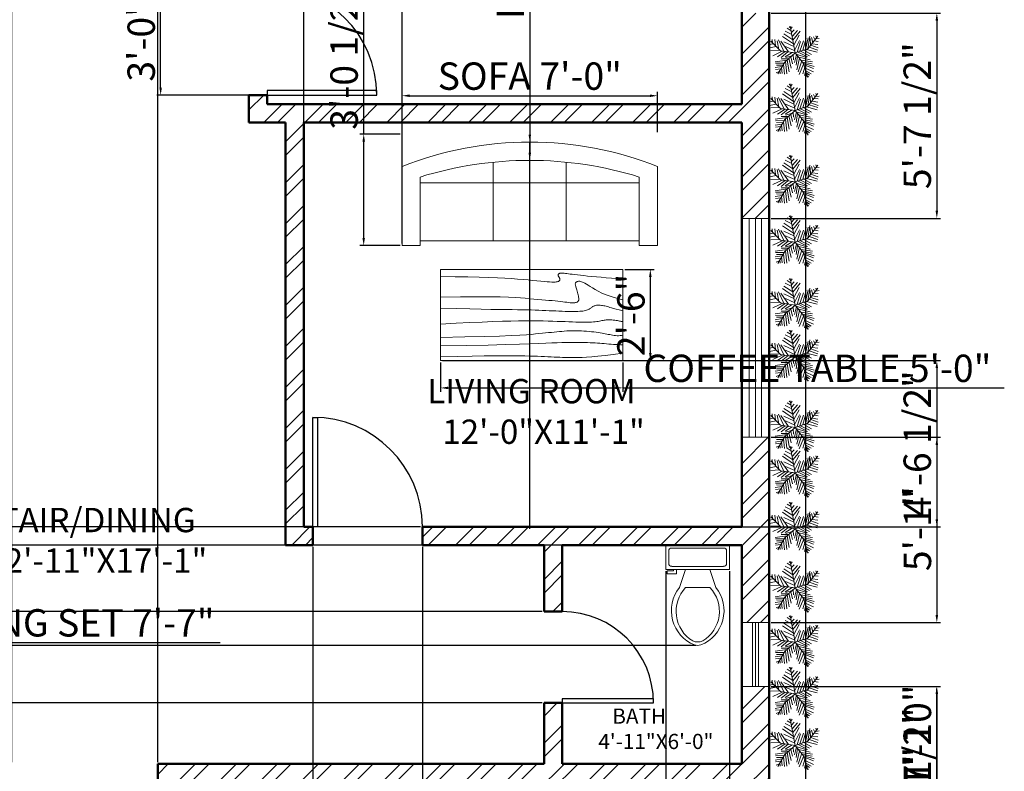
# Model space of a CAD drawing. Units: inches. Extents: x 176 to 806, y 915 to 1663.
# Tile 4 of 5: x 482 to 806, y 1198 to 1445. Entities that reach past the tile are written whole.
import ezdxf

# ---------------------------------------------------------------- set-up
doc = ezdxf.new("R2010")
doc.units = ezdxf.units.IN
for name, color, linetype, lineweight in [('A-ANNO-DIMS', 2, 'Continuous', 18), ('A-AREA-IDEN', 7, 'Continuous', 18), ('A-DOOR', 4, 'Continuous', 25), ('A-FLOR-FIXT', 9, 'Continuous', 18), ('A-FURN', 8, 'Continuous', 18), ('A-WALL', 7, 'Continuous', 50), ('A-WALL-PATT', 252, 'Continuous', 13), ('C-PROP', 8, 'Continuous', 25), ('L-PLNT', 3, 'Continuous', 13)]:
    doc.layers.add(name, color=color, linetype=linetype, lineweight=lineweight)
doc.layers.add('A-GLAZ', color=244, linetype='Continuous', lineweight=18, true_color=0x991b1e)
doc.styles.get("Standard").update_dxf_attribs({"font": 'arial.ttf'})
doc.dimstyles.new('ISO-25', dxfattribs={"dimtxt": 9, "dimasz": 2.5, "dimexe": 1.25, "dimexo": 0.625, "dimtad": 1, "dimlunit": 3, "dimtxsty": 'Standard', "dimcen": 2.5, "dimadec": 0, "dimazin": 0, "dimtfac": 1, "dimtmove": 0, "dimatfit": 3, "dimfxl": 1, "dimarcsym": 0})

# ---------------------------------------------------------------- blocks, each defined once
blk = doc.blocks.new('*U3')
for p, q in [((0, 0), (0, -6)), ((-40, 0), (-40, -6))]:
    blk.add_line(p, q)
blk.add_lwpolyline([(0, 0), (0, 40), (-1.75, 40), (-1.75, 0)], close=True)
blk.add_arc((0, 0), 40, 90, 180)
blk = doc.blocks.new('*U5')
for p, q in [((0, 0), (0, -6)), ((40, 0), (40, -6))]:
    blk.add_line(p, q)
blk.add_lwpolyline([(0, 0), (0, 40), (1.75, 40), (1.75, 0)], close=True)
blk.add_arc((0, 0), 40, 0, 90)
blk = doc.blocks.new('*U6')
for p, q in [((0, 0), (0, 6)), ((40, 0), (40, 6))]:
    blk.add_line(p, q)
blk.add_lwpolyline([(0, 0), (0, -40), (1.75, -40), (1.75, 0)], close=True)
blk.add_arc((0, 0), 40, 270, 0)
blk = doc.blocks.new('*U8')
for p, q in [((-7.288, 39.707), (-21.778, 46.673)), ((-8.737, 47.138), (-17.069, 52.711)), ((-10.186, 53.64), (-13.084, 55.962)), ((0, 0), (-10.5, 57)), ((-9.099, 51.782), (-6.563, 55.962)), ((-7.65, 43.423), (-2.578, 49.46)), ((-5.839, 35.992), (4.667, 48.067)), ((-5.114, 27.632), (10.463, 46.673)), ((-31.5, 4.5), (-52.5, 25.5)), ((-48.585, 21.131), (-49.309, 29.026)), ((-43.513, 28.561), (-42.427, 15.558)), ((-38.442, 26.239), (-34.819, 7.663)), ((-35.544, 28.097), (-24.314, 3.947)), ((-14.533, 2.09), (-30.834, 25.31)), ((-3.665, 19.273), (-27.574, 35.527)), ((-5.114, 28.097), (-24.676, 40.636)), ((-24.314, 23.917), (-2.941, 13.7)), ((-2.941, 16.486), (8.652, 37.85)), ((-1.129, 6.734), (9.014, 26.704)), ((3.942, 1.625), (11.187, 24.381)), ((10.101, 3.483), (17.708, 26.239)), ((16.259, 5.805), (23.142, 31.348)), ((22.055, 7.198), (27.489, 32.277)), ((27, 9), (48, 36)), ((27.127, 9.056), (31.112, 35.992)), ((31.836, 30.883), (32.561, 16.486)), ((35.096, 32.741), (37.27, 22.524)), ((38.719, 34.134), (41.979, 28.561)), ((40.53, 25.775), (48.862, 24.846)), ((43.791, 29.954), (51.036, 30.883)), ((44.153, 36.456), (45.239, 32.741)), ((-47.498, 19.737), (-55.83, 18.344)), ((-40.615, 13.7), (-55.105, 10.913)), ((-33.37, 6.269), (-52.207, 5.34)), ((-28.299, 3.483), (-47.86, -5.805)), ((-21.416, 3.018), (-38.079, -8.128)), ((0, 0), (-31.5, 4.5)), ((-15.982, 2.09), (-30.11, -9.521)), ((0, 0), (-22.5, -19.5)), ((-6.563, 1.161), (-21.416, -8.128)), ((-20.691, 13.7), (-1.129, 4.876)), ((0, 0), (27, 9)), ((0, 0), (18, -22.5)), ((6.478, 1.625), (26.04, -8.592)), ((11.187, 3.483), (30.749, -5.805)), ((18.07, 5.805), (35.096, -3.483)), ((24.229, 7.663), (46.688, 1.625)), ((29.662, 12.307), (48.137, 6.269)), ((33.285, 16.486), (48.862, 10.913)), ((36.183, 19.737), (48.137, 17.88)), ((-17.431, -15.094), (-42.789, -18.809)), ((-22.5, -19.5), (-37.5, -45)), ((-15.257, -12.772), (-30.11, -12.772)), ((-20.691, -18.345), (-17.793, -44.352)), ((-6.563, -5.805), (-19.967, -9.985)), ((-17.069, -15.094), (-12.721, -40.172)), ((-13.446, -11.378), (-8.737, -32.741)), ((-9.461, -8.592), (-6.201, -23.453)), ((-4.752, -3.483), (-3.665, -14.629)), ((2.493, -3.019), (-1.491, -20.202)), ((1.769, -2.555), (24.229, -9.521)), ((5.029, -6.27), (2.131, -25.775)), ((9.014, -11.378), (3.58, -35.992)), ((14.085, -16.951), (6.478, -40.172)), ((7.565, -9.056), (32.198, -14.629)), ((12.274, -15.094), (36.907, -18.809)), ((16.259, -19.738), (36.183, -22.989)), ((-28.299, -29.026), (-42.789, -31.348)), ((-24.314, -21.596), (-42.427, -22.06)), ((-30.834, -34.135), (-42.427, -35.528)), ((-34.457, -39.708), (-40.978, -42.494)), ((-26.849, -26.24), (-40.253, -25.775)), ((-32.646, -36.921), (-31.921, -44.352)), ((-29.023, -30.884), (-27.936, -43.887)), ((-25.038, -23.918), (-22.865, -45.281)), ((18.07, -22.524), (8.289, -45.745)), ((20.244, -30.419), (15.897, -44.816)), ((18, -22.5), (27, -52.5)), ((18.433, -22.524), (40.53, -29.026)), ((19.157, -25.311), (38.719, -33.206)), ((22.78, -37.85), (19.519, -48.532)), ((21.331, -32.741), (39.081, -40.636)), ((22.78, -38.314), (34.372, -44.816)), ((24.591, -45.745), (23.142, -50.854)), ((24.591, -43.423), (30.749, -47.603)), ((26.764, -49.925), (28.213, -50.854))]:
    blk.add_line(p, q)
blk = doc.blocks.new('*U13')
for p, q in [((9.5, -6), (9.5, -2)), ((-10, -8.5), (-8, -8.5)), ((-10, -9.5), (-10, -8.5)), ((-7, -9.5), (-10, -9.5)), ((-8, -8.5), (-8, -8)), ((-7, -8), (-7, -9.5)), ((-4, -8), (-6, -14)), ((4, -8), (6, -14)), ((4, -14), (-4, -14))]:
    blk.add_line(p, q)
blk.add_lwpolyline([(10.5, -8), (10.5, 0), (-10.5, 0), (-10.5, -8)], close=True)
for points in [[(-9.5, -2), (-9.5, -6)], [(8.5, -1), (-8.5, -1)], [(-8.5, -7), (8.5, -7)]]:
    blk.add_lwpolyline(points)
for centre, radius, start, end in [((-8.62, -1.88), 0.884, 81.8699, 188.1301), ((8.62, -1.88), 0.884, 351.8699, 98.1301), ((-8.62, -6.12), 0.884, 171.8699, 278.1301), ((8.62, -6.12), 0.884, 261.8699, 8.1301), ((3.52, -21.58), 12.17, 141.4691, 247.9714), ((4.2, -21.82), 11.33, 136.3677, 238.9468), ((-3.52, -21.58), 12.17, 292.0284, 38.5307), ((-4.2, -21.82), 11.33, 301.053, 43.6321), ((0, -27.88), 4, 245.7318, 294.2682), ((0, -29), 4, 254.8605, 285.1395)]:
    blk.add_arc(centre, radius, start, end)
blk = doc.blocks.new('Sofa - Roundback 7 ft.')
for p, q in [((-12.00002, -32.4421), (-12.00003, -6.5971)), ((11.99997, -32.4421), (11.99998, -6.5971)), ((-36.000027, -34), (-36.000027, -11.4696)), ((35.99998, -34), (35.99998, -11.4696)), ((-35.999844, -13.3819), (35.9998, -13.3819)), ((-36.000027, -32.4421), (35.99998, -32.4421))]:
    blk.add_line(p, q)
for points in [[(-36.000027, -34), (-42.000027, -34), (-42.000027, -8)], [(41.99998, -8), (41.99998, -34), (35.99998, -34)]]:
    blk.add_lwpolyline(points)
for centre, radius, start, end in [((0, -114.25), 114.25, 68.43141, 111.5686), ((-0.00001, -127.1968), 121.1968, 72.72033, 107.2797)]:
    blk.add_arc(centre, radius, start, end)
blk = doc.blocks.new('Table - Rectangular Woodgrain 60 x 30 in.')
for p, q in [((0, 0), (0, -30)), ((60, 0), (0, 0)), ((60, -30), (60, 0)), ((0, -30), (60, -30))]:
    blk.add_line(p, q)
for points in [[(0, -2.4), (4.8155, -2.418), (9.0302, -2.4688), (12.709, -2.5477), (15.9167, -2.65), (18.7181, -2.7711), (21.1781, -2.9063), (23.3616, -3.0508), (25.3333, -3.2), (27.1477, -3.3495), (28.8172, -3.4958), (30.3437, -3.636), (31.7291, -3.7667), (32.9756, -3.8849), (34.0849, -3.9875), (35.059, -4.0714), (35.9, -4.1334), (36.6114, -4.1711), (37.2041, -4.1854), (37.6906, -4.1779), (38.0833, -4.15), (38.3948, -4.1034), (38.6375, -4.0396), (38.8239, -3.9602), (38.9666, -3.8667), (39.0764, -3.7608), (39.1573, -3.6448), (39.2116, -3.521), (39.2416, -3.3917), (39.2498, -3.2593), (39.2385, -3.1261), (39.21, -2.9944), (39.1666, -2.8667), (39.111, -2.7447), (39.0468, -2.6281), (38.978, -2.5163), (38.9083, -2.4083), (38.8418, -2.3035), (38.7823, -2.201), (38.7337, -2.1001), (38.7, -2), (38.6844, -1.9003), (38.6875, -1.8021), (38.7094, -1.707), (38.75, -1.6167), (38.8094, -1.5326), (38.8875, -1.4563), (38.9844, -1.3893), (39.1, -1.3333), (39.2351, -1.2896), (39.3937, -1.2583), (39.5804, -1.2396), (39.8, -1.2333), (40.057, -1.2396), (40.3562, -1.2583), (40.7023, -1.2896), (41.1, -1.3333), (41.5547, -1.3895), (42.0755, -1.4573), (42.6721, -1.5361), (43.3542, -1.625), (44.1316, -1.7233), (45.014, -1.8302), (46.0114, -1.9449), (47.1333, -2.0667), (48.3862, -2.1947), (49.7625, -2.3281), (51.2513, -2.4663), (52.8416, -2.6083), (54.5226, -2.7535), (56.2833, -2.9011), (58.1127, -3.0501), (60, -3.2)], [(0, -9.2), (6.5759, -9.0858), (11.9385, -9.0365), (16.2527, -9.0418), (19.6833, -9.0917), (22.3952, -9.1759), (24.5531, -9.2844), (26.322, -9.4069), (27.8666, -9.5333), (29.3241, -9.6553), (30.7203, -9.7719), (32.0532, -9.8837), (33.3208, -9.9917), (34.5213, -10.0965), (35.6526, -10.199), (36.7128, -10.2999), (37.7, -10.4), (38.6129, -10.4996), (39.4531, -10.5969), (40.223, -10.6895), (40.925, -10.775), (41.5613, -10.8512), (42.1344, -10.9156), (42.6465, -10.966), (43.1, -11), (43.4976, -11.0158), (43.8437, -11.0136), (44.143, -10.9942), (44.4, -10.9583), (44.6195, -10.9069), (44.8062, -10.8406), (44.9648, -10.7603), (45.1, -10.6667), (45.2155, -10.5598), (45.3114, -10.4365), (45.3871, -10.2929), (45.4416, -10.125), (45.4743, -9.929), (45.4844, -9.7011), (45.4709, -9.4371), (45.4333, -9.1333), (45.3716, -8.7883), (45.2896, -8.4104), (45.1919, -8.0107), (45.0833, -7.6), (44.9685, -7.1893), (44.8521, -6.7896), (44.7388, -6.4117), (44.6333, -6.0667), (44.54, -5.7628), (44.4614, -5.4979), (44.4001, -5.2675), (44.3583, -5.0667), (44.3384, -4.8909), (44.3427, -4.7354), (44.3736, -4.5956), (44.4333, -4.4667), (44.5236, -4.3453), (44.6427, -4.2333), (44.7884, -4.1339), (44.9583, -4.05), (45.1501, -3.9849), (45.3614, -3.9417), (45.59, -3.9234), (45.8333, -3.9333), (46.0915, -3.9749), (46.3734, -4.0531), (46.6906, -4.1736), (47.0542, -4.3417), (47.4756, -4.5629), (47.9661, -4.8427), (48.5372, -5.1866), (49.2, -5.6), (49.9676, -6.0844), (50.8594, -6.625), (51.8965, -7.2031), (53.1, -7.8), (54.491, -8.3969), (56.0906, -8.975), (57.9199, -9.5156), (60, -10)], [(0, -12.8), (5.1847, -12.9322), (9.6213, -13.0323), (13.3963, -13.1059), (16.5958, -13.1583), (19.3063, -13.1952), (21.614, -13.2219), (23.6054, -13.2439), (25.3666, -13.2667), (26.9728, -13.2947), (28.4531, -13.3281), (29.8256, -13.3663), (31.1083, -13.4083), (32.3191, -13.4535), (33.476, -13.501), (34.597, -13.5501), (35.7, -13.6), (36.7984, -13.6497), (37.8875, -13.6979), (38.9578, -13.743), (40, -13.7833), (41.0047, -13.8174), (41.9625, -13.8438), (42.864, -13.8607), (43.7, -13.8667), (44.4631, -13.8604), (45.1552, -13.8417), (45.7801, -13.8104), (46.3416, -13.7667), (46.8439, -13.7104), (47.2906, -13.6417), (47.6858, -13.5604), (48.0333, -13.4667), (48.3375, -13.3608), (48.6042, -13.2448), (48.8396, -13.121), (49.05, -12.9917), (49.2417, -12.8593), (49.4208, -12.7261), (49.5937, -12.5944), (49.7667, -12.4667), (49.9452, -12.3451), (50.1323, -12.2313), (50.3303, -12.1268), (50.5416, -12.0333), (50.7686, -11.9524), (51.0135, -11.8854), (51.2788, -11.8341), (51.5666, -11.8), (51.8785, -11.7843), (52.2116, -11.7865), (52.562, -11.8059), (52.926, -11.8417), (53.2998, -11.8931), (53.6795, -11.9594), (54.0614, -12.0397), (54.4416, -12.1333), (54.8223, -12.2401), (55.2293, -12.3625), (55.6942, -12.5037), (56.2489, -12.6667), (56.9251, -12.8547), (57.7545, -13.0708), (58.7689, -13.3182), (60, -13.6)], [(0, -18), (5.124, -17.7273), (9.6609, -17.5057), (13.6705, -17.3303), (17.2125, -17.1958), (20.3467, -17.0973), (23.1328, -17.0297), (25.6307, -16.9878), (27.9, -16.9667), (29.9928, -16.9617), (31.9302, -16.9703), (33.7254, -16.9907), (35.3917, -17.0208), (36.9423, -17.0588), (38.3906, -17.1026), (39.7499, -17.1503), (41.0333, -17.2), (42.2519, -17.2496), (43.4073, -17.2969), (44.4986, -17.3395), (45.525, -17.375), (46.4858, -17.4012), (47.3802, -17.4156), (48.2074, -17.416), (48.9667, -17.4), (49.6583, -17.3662), (50.2872, -17.3167), (50.8595, -17.2547), (51.3812, -17.1833), (51.8584, -17.1057), (52.2971, -17.025), (52.7034, -16.9443), (53.0833, -16.8667), (53.443, -16.7951), (53.789, -16.7313), (54.128, -16.6768), (54.4666, -16.6334), (54.8115, -16.6024), (55.1693, -16.5854), (55.5465, -16.5841), (55.95, -16.6), (56.3828, -16.6337), (56.8346, -16.6823), (57.2915, -16.7418), (57.7396, -16.8084), (58.165, -16.878), (58.5539, -16.9469), (58.8924, -17.0111), (59.1666, -17.0667), (59.3679, -17.1107), (59.5078, -17.1438), (59.6032, -17.1675), (59.6708, -17.1833), (59.7275, -17.193), (59.7901, -17.1979), (59.8753, -17.1998), (60, -17.2)], [(0, -22.4), (8.0098, -22.2501), (14.4094, -22.1011), (19.4168, -21.9535), (23.25, -21.8083), (26.1269, -21.6663), (28.2656, -21.5281), (29.884, -21.3947), (31.2, -21.2667), (32.3967, -21.1448), (33.5172, -21.0292), (34.5697, -20.9198), (35.5625, -20.8167), (36.5037, -20.7198), (37.4015, -20.6292), (38.2642, -20.5448), (39.1, -20.4667), (39.9164, -20.3951), (40.7187, -20.3313), (41.5117, -20.2768), (42.3, -20.2333), (43.0883, -20.2024), (43.8812, -20.1854), (44.6836, -20.1841), (45.5, -20.2), (46.3328, -20.234), (47.1747, -20.2844), (48.0163, -20.3488), (48.8479, -20.425), (49.66, -20.5106), (50.4429, -20.6031), (51.1872, -20.7004), (51.8833, -20.8), (52.5246, -20.8999), (53.1166, -20.9995), (53.6681, -21.0983), (54.1875, -21.1958), (54.6834, -21.2919), (55.1646, -21.3859), (55.6394, -21.4777), (56.1167, -21.5667), (56.6028, -21.6515), (57.0961, -21.7266), (57.5929, -21.7852), (58.0896, -21.8208), (58.5823, -21.8268), (59.0674, -21.7964), (59.5412, -21.723), (60, -21.6)], [(0, -25.2), (8.6355, -25.0504), (15.7026, -24.9031), (21.4049, -24.7606), (25.9458, -24.625), (29.529, -24.4988), (32.3578, -24.3844), (34.6359, -24.284), (36.5667, -24.2), (38.3213, -24.1341), (39.9417, -24.0854), (41.437, -24.0523), (42.8167, -24.0333), (44.0901, -24.0268), (45.2667, -24.0313), (46.3557, -24.0451), (47.3667, -24.0667), (48.309, -24.0947), (49.1928, -24.1287), (50.0284, -24.168), (50.826, -24.2125), (51.5959, -24.2617), (52.3483, -24.3151), (53.0935, -24.3725), (53.8417, -24.4334), (54.6009, -24.497), (55.3699, -24.561), (56.1454, -24.6226), (56.9239, -24.6792), (57.7021, -24.7279), (58.4764, -24.7662), (59.2435, -24.7911), (60, -24.8)], [(0, -28.8), (5.6867, -28.6681), (10.45, -28.5698), (14.407, -28.5012), (17.675, -28.4584), (20.3711, -28.4374), (22.6125, -28.4344), (24.5164, -28.4455), (26.2, -28.4667), (27.762, -28.4947), (29.2276, -28.5281), (30.6033, -28.5663), (31.8958, -28.6084), (33.1118, -28.6535), (34.2578, -28.7011), (35.3405, -28.7501), (36.3666, -28.8), (37.3443, -28.8497), (38.288, -28.8974), (39.2137, -28.9412), (40.1375, -28.9792), (41.0753, -29.0093), (42.0432, -29.0297), (43.0572, -29.0384), (44.1333, -29.0333), (45.2936, -29.0114), (46.5843, -28.9641), (48.0579, -28.8816), (49.7666, -28.7542), (51.7629, -28.5721), (54.0989, -28.3255), (56.8272, -28.0048), (60, -27.6)]]:
    blk.add_lwpolyline(points)
blk = doc.blocks.new('WIN-GLAZING-72IN')
for p, q in [((0, 2), (72, 2)), ((0, 0), (72, 0)), ((0, -2), (72, -2))]:
    blk.add_line(p, q)
blk = doc.blocks.new('WIN-GLAZING-21IN')
for p, q in [((0, 1), (21, 1)), ((0, 0), (21, 0)), ((0, -1), (21, -1))]:
    blk.add_line(p, q)
blk = doc.blocks.new('*D34')
at = {"layer": 'A-ANNO-DIMS', "color": 0, "lineweight": -2, "transparency": 16777216}
for p, q in [((354.6, 1253.2), (354.6, 1238.92)), ((445.6, 1253.2), (445.6, 1238.92)), ((357.1, 1240.17), (443.1, 1240.17)), ((445.6, 1240.17), (548.27, 1240.17))]:
    blk.add_line(p, q, dxfattribs=at)
at = {"layer": 'A-ANNO-DIMS', "color": 0, "transparency": 16777216}
for points in [[(357.1, 1240.59), (357.1, 1239.75), (354.6, 1240.17)], [(443.1, 1240.59), (443.1, 1239.75), (445.6, 1240.17)]]:
    blk.add_solid(points, dxfattribs=at)
at = {"layer": 'Defpoints', "color": 0, "transparency": 16777216}
for p in [(354.6, 1253.82), (445.6, 1253.82), (445.6, 1240.17)]:
    blk.add_point(p, dxfattribs=at)
at = {"layer": 'A-ANNO-DIMS', "color": 0, "transparency": 16777216, "insert": (498.18, 1245.45), "char_height": 9, "attachment_point": 5}
blk.add_mtext('DINING SET 7\'-7"', dxfattribs=at)
blk = doc.blocks.new('*D36')
at = {"layer": 'A-ANNO-DIMS', "color": 0, "lineweight": -2, "transparency": 16777216}
for p, q in [((608.02, 1408.04), (608.02, 1421.26)), ((692.02, 1408.04), (692.02, 1421.26)), ((610.52, 1420.01), (689.52, 1420.01))]:
    blk.add_line(p, q, dxfattribs=at)
at = {"layer": 'A-ANNO-DIMS', "color": 0, "transparency": 16777216}
for points in [[(610.52, 1420.43), (610.52, 1419.59), (608.02, 1420.01)], [(689.52, 1420.43), (689.52, 1419.59), (692.02, 1420.01)]]:
    blk.add_solid(points, dxfattribs=at)
at = {"layer": 'Defpoints', "color": 0, "transparency": 16777216}
for p in [(692.02, 1420.01), (608.02, 1407.41), (692.02, 1407.41)]:
    blk.add_point(p, dxfattribs=at)
at = {"layer": 'A-ANNO-DIMS', "color": 0, "transparency": 16777216, "insert": (650.02, 1425.29), "char_height": 9, "attachment_point": 5}
blk.add_mtext('SOFA 7\'-0"', dxfattribs=at)
blk = doc.blocks.new('*D37')
at = {"layer": 'A-ANNO-DIMS', "color": 0, "lineweight": -2, "transparency": 16777216}
for p, q in [((595.42, 1407.41), (595.42, 1456.05)), ((607.4, 1407.41), (594.17, 1407.41)), ((595.42, 1373.24), (595.42, 1404.91)), ((607.4, 1370.74), (594.17, 1370.74))]:
    blk.add_line(p, q, dxfattribs=at)
at = {"layer": 'A-ANNO-DIMS', "color": 0, "transparency": 16777216}
for points in [[(595.01, 1404.91), (595.84, 1404.91), (595.42, 1407.41)], [(595.01, 1373.24), (595.84, 1373.24), (595.42, 1370.74)]]:
    blk.add_solid(points, dxfattribs=at)
at = {"layer": 'Defpoints', "color": 0, "transparency": 16777216}
for p in [(595.42, 1407.41), (608.02, 1407.41), (608.02, 1370.74)]:
    blk.add_point(p, dxfattribs=at)
at = {"layer": 'A-ANNO-DIMS', "color": 0, "transparency": 16777216, "insert": (590.14, 1432.98), "char_height": 9, "attachment_point": 5, "rotation": 90}
blk.add_mtext('3\'-0 1/2"', dxfattribs=at)
blk = doc.blocks.new('*D38')
at = {"layer": 'A-ANNO-DIMS', "color": 0, "lineweight": -2, "transparency": 16777216}
for p, q in [((620.66, 1332.28), (620.66, 1322.65)), ((680.66, 1332.28), (680.66, 1322.65)), ((623.16, 1323.9), (678.16, 1323.9)), ((680.66, 1323.9), (806.03, 1323.9))]:
    blk.add_line(p, q, dxfattribs=at)
at = {"layer": 'A-ANNO-DIMS', "color": 0, "transparency": 16777216}
for points in [[(623.16, 1324.32), (623.16, 1323.48), (620.66, 1323.9)], [(678.16, 1324.32), (678.16, 1323.48), (680.66, 1323.9)]]:
    blk.add_solid(points, dxfattribs=at)
at = {"layer": 'Defpoints', "color": 0, "transparency": 16777216}
for p in [(620.66, 1332.9), (680.66, 1332.9), (680.66, 1323.9)]:
    blk.add_point(p, dxfattribs=at)
at = {"layer": 'A-ANNO-DIMS', "color": 0, "transparency": 16777216, "insert": (744.59, 1329.18), "char_height": 9, "attachment_point": 5}
blk.add_mtext('COFFEE TABLE 5\'-0"', dxfattribs=at)
blk = doc.blocks.new('*D39')
at = {"layer": 'A-ANNO-DIMS', "color": 0, "lineweight": -2, "transparency": 16777216}
for p, q in [((681.28, 1362.9), (690.91, 1362.9)), ((689.66, 1335.4), (689.66, 1360.4)), ((681.28, 1332.9), (690.91, 1332.9))]:
    blk.add_line(p, q, dxfattribs=at)
at = {"layer": 'A-ANNO-DIMS', "color": 0, "transparency": 16777216}
for points in [[(689.24, 1360.4), (690.07, 1360.4), (689.66, 1362.9)], [(689.24, 1335.4), (690.07, 1335.4), (689.66, 1332.9)]]:
    blk.add_solid(points, dxfattribs=at)
at = {"layer": 'Defpoints', "color": 0, "transparency": 16777216}
for p in [(680.66, 1362.9), (689.66, 1362.9), (680.66, 1332.9)]:
    blk.add_point(p, dxfattribs=at)
at = {"layer": 'A-ANNO-DIMS', "color": 0, "transparency": 16777216, "insert": (684.44, 1347.9), "char_height": 9, "attachment_point": 5, "rotation": 90}
blk.add_mtext('2\'-6"', dxfattribs=at)
blk = doc.blocks.new('*D45')
at = {"layer": 'A-ANNO-DIMS', "color": 0, "lineweight": -2, "transparency": 16777216}
for p, q in [((729.33, 1447.21), (785.1, 1447.21)), ((783.85, 1444.71), (783.85, 1382.17)), ((729.33, 1379.67), (785.1, 1379.67))]:
    blk.add_line(p, q, dxfattribs=at)
at = {"layer": 'A-ANNO-DIMS', "color": 0, "transparency": 16777216}
for points in [[(783.43, 1444.71), (784.27, 1444.71), (783.85, 1447.21)], [(783.43, 1382.17), (784.27, 1382.17), (783.85, 1379.67)]]:
    blk.add_solid(points, dxfattribs=at)
at = {"layer": 'Defpoints', "color": 0, "transparency": 16777216}
for p in [(728.7, 1447.21), (728.7, 1379.67), (783.85, 1379.67)]:
    blk.add_point(p, dxfattribs=at)
at = {"layer": 'A-ANNO-DIMS', "color": 0, "transparency": 16777216, "insert": (778.57, 1413.44), "char_height": 9, "attachment_point": 5, "rotation": 90}
blk.add_mtext('5\'-7 1/2"', dxfattribs=at)
blk = doc.blocks.new('*D46')
at = {"layer": 'A-ANNO-DIMS', "color": 0, "lineweight": -2, "transparency": 16777216}
for p, q in [((729.33, 1307.67), (785.1, 1307.67)), ((783.85, 1305.17), (783.85, 1249.21)), ((729.33, 1246.71), (785.1, 1246.71))]:
    blk.add_line(p, q, dxfattribs=at)
at = {"layer": 'A-ANNO-DIMS', "color": 0, "transparency": 16777216}
for points in [[(783.43, 1305.17), (784.27, 1305.17), (783.85, 1307.67)], [(783.43, 1249.21), (784.27, 1249.21), (783.85, 1246.71)]]:
    blk.add_solid(points, dxfattribs=at)
at = {"layer": 'Defpoints', "color": 0, "transparency": 16777216}
for p in [(728.7, 1307.67), (728.7, 1246.71), (783.85, 1246.71)]:
    blk.add_point(p, dxfattribs=at)
at = {"layer": 'A-ANNO-DIMS', "color": 0, "transparency": 16777216, "insert": (778.63, 1277.19), "char_height": 9, "attachment_point": 5, "rotation": 90}
blk.add_mtext('5\'-1"', dxfattribs=at)
blk = doc.blocks.new('*D47')
at = {"layer": 'A-ANNO-DIMS', "color": 0, "lineweight": -2, "transparency": 16777216}
for p, q in [((729.33, 1225.71), (785.1, 1225.71)), ((783.85, 1223.21), (783.85, 1161.23)), ((729.33, 1158.73), (785.1, 1158.73))]:
    blk.add_line(p, q, dxfattribs=at)
at = {"layer": 'A-ANNO-DIMS', "color": 0, "transparency": 16777216}
for points in [[(783.43, 1223.21), (784.27, 1223.21), (783.85, 1225.71)], [(783.43, 1161.23), (784.27, 1161.23), (783.85, 1158.73)]]:
    blk.add_solid(points, dxfattribs=at)
at = {"layer": 'Defpoints', "color": 0, "transparency": 16777216}
for p in [(728.7, 1225.71), (728.7, 1158.73), (783.85, 1158.73)]:
    blk.add_point(p, dxfattribs=at)
at = {"layer": 'A-ANNO-DIMS', "color": 0, "transparency": 16777216, "insert": (778.65, 1192.22), "char_height": 9, "attachment_point": 5, "rotation": 90}
blk.add_mtext('5\'-7"', dxfattribs=at)
blk = doc.blocks.new('*D52')
at = {"layer": 'A-ANNO-DIMS', "color": 0, "lineweight": -2, "transparency": 16777216}
for p, q in [((479.7, 1200.83), (479.7, 1645.51)), ((527.7, 1200.83), (527.7, 1645.51)), ((482.2, 1644.26), (525.2, 1644.26))]:
    blk.add_line(p, q, dxfattribs=at)
at = {"layer": 'A-ANNO-DIMS', "color": 0, "transparency": 16777216}
for points in [[(482.2, 1644.67), (482.2, 1643.84), (479.7, 1644.26)], [(525.2, 1644.67), (525.2, 1643.84), (527.7, 1644.26)]]:
    blk.add_solid(points, dxfattribs=at)
at = {"layer": 'Defpoints', "color": 0, "transparency": 16777216}
for p in [(527.7, 1644.26), (479.7, 1200.21), (527.7, 1200.21)]:
    blk.add_point(p, dxfattribs=at)
at = {"layer": 'A-ANNO-DIMS', "color": 0, "transparency": 16777216, "insert": (503.7, 1649.48), "char_height": 9, "attachment_point": 5}
blk.add_mtext('4\'-0"', dxfattribs=at)
blk = doc.blocks.new('*D54')
at = {"layer": 'A-ANNO-DIMS', "color": 0, "lineweight": -2, "transparency": 16777216}
for p, q in [((247.1, 1280.71), (247.1, 1283.21)), ((614.08, 1278.21), (245.85, 1278.21)), ((247.1, 1278.21), (247.1, 1272.21)), ((614.08, 1272.21), (245.85, 1272.21)), ((247.1, 1269.71), (247.1, 1242.03))]:
    blk.add_line(p, q, dxfattribs=at)
at = {"layer": 'A-ANNO-DIMS', "color": 0, "transparency": 16777216}
for points in [[(246.68, 1280.71), (247.52, 1280.71), (247.1, 1278.21)], [(246.68, 1269.71), (247.52, 1269.71), (247.1, 1272.21)]]:
    blk.add_solid(points, dxfattribs=at)
at = {"layer": 'Defpoints', "color": 0, "transparency": 16777216}
for p in [(614.7, 1278.21), (247.1, 1272.21), (614.7, 1272.21)]:
    blk.add_point(p, dxfattribs=at)
at = {"layer": 'A-ANNO-DIMS', "color": 0, "transparency": 16777216, "insert": (241.88, 1254.62), "char_height": 9, "attachment_point": 5, "rotation": 90}
blk.add_mtext('0\'-6"', dxfattribs=at)
blk = doc.blocks.new('*D58')
at = {"layer": 'A-ANNO-DIMS', "color": 0, "lineweight": -2, "transparency": 16777216}
for p, q in [((654.08, 1250.31), (245.85, 1250.31)), ((247.1, 1222.81), (247.1, 1247.81)), ((654.08, 1220.31), (245.85, 1220.31))]:
    blk.add_line(p, q, dxfattribs=at)
at = {"layer": 'A-ANNO-DIMS', "color": 0, "transparency": 16777216}
for points in [[(246.68, 1247.81), (247.52, 1247.81), (247.1, 1250.31)], [(246.68, 1222.81), (247.52, 1222.81), (247.1, 1220.31)]]:
    blk.add_solid(points, dxfattribs=at)
at = {"layer": 'Defpoints', "color": 0, "transparency": 16777216}
for p in [(247.1, 1250.31), (654.7, 1250.31), (654.7, 1220.31)]:
    blk.add_point(p, dxfattribs=at)
at = {"layer": 'A-ANNO-DIMS', "color": 0, "transparency": 16777216, "insert": (241.88, 1235.31), "char_height": 9, "attachment_point": 5, "rotation": 90}
blk.add_mtext('2\'-6"', dxfattribs=at)
blk = doc.blocks.new('*D60')
at = {"layer": 'A-ANNO-DIMS', "color": 0, "lineweight": -2, "transparency": 16777216}
for p, q in [((578.7, 1271.58), (578.7, 983.8)), ((614.7, 1271.58), (614.7, 983.8)), ((581.2, 985.05), (612.2, 985.05))]:
    blk.add_line(p, q, dxfattribs=at)
at = {"layer": 'A-ANNO-DIMS', "color": 0, "transparency": 16777216}
for points in [[(581.2, 985.47), (581.2, 984.64), (578.7, 985.05)], [(612.2, 985.47), (612.2, 984.64), (614.7, 985.05)]]:
    blk.add_solid(points, dxfattribs=at)
at = {"layer": 'Defpoints', "color": 0, "transparency": 16777216}
for p in [(578.7, 1272.21), (614.7, 1272.21), (614.7, 985.05)]:
    blk.add_point(p, dxfattribs=at)
at = {"layer": 'A-ANNO-DIMS', "color": 0, "transparency": 16777216, "insert": (596.7, 990.28), "char_height": 9, "attachment_point": 5}
blk.add_mtext('3\'-0"', dxfattribs=at)
blk = doc.blocks.new('*D63')
at = {"layer": 'A-ANNO-DIMS', "color": 0, "lineweight": -2, "transparency": 16777216}
for p, q in [((783.85, 1169.12), (783.85, 1217.75)), ((334.37, 1169.12), (785.1, 1169.12)), ((783.85, 1129.89), (783.85, 1166.62)), ((334.37, 1127.39), (785.1, 1127.39))]:
    blk.add_line(p, q, dxfattribs=at)
at = {"layer": 'A-ANNO-DIMS', "color": 0, "transparency": 16777216}
for points in [[(783.43, 1166.62), (784.27, 1166.62), (783.85, 1169.12)], [(783.43, 1129.89), (784.27, 1129.89), (783.85, 1127.39)]]:
    blk.add_solid(points, dxfattribs=at)
at = {"layer": 'Defpoints', "color": 0, "transparency": 16777216}
for p in [(333.74, 1169.12), (783.85, 1169.12), (333.74, 1127.39)]:
    blk.add_point(p, dxfattribs=at)
at = {"layer": 'A-ANNO-DIMS', "color": 0, "transparency": 16777216, "insert": (778.57, 1194.68), "char_height": 9, "attachment_point": 5, "rotation": 90}
blk.add_mtext('3\'-5 1/2"', dxfattribs=at)
blk = doc.blocks.new('*D64')
at = {"layer": 'A-ANNO-DIMS', "color": 0, "lineweight": -2, "transparency": 16777216}
for p, q in [((563.08, 1456.21), (527.4, 1456.21)), ((528.65, 1422.71), (528.65, 1453.71)), ((563.08, 1420.21), (527.4, 1420.21))]:
    blk.add_line(p, q, dxfattribs=at)
at = {"layer": 'A-ANNO-DIMS', "color": 0, "transparency": 16777216}
for points in [[(528.24, 1453.71), (529.07, 1453.71), (528.65, 1456.21)], [(528.24, 1422.71), (529.07, 1422.71), (528.65, 1420.21)]]:
    blk.add_solid(points, dxfattribs=at)
at = {"layer": 'Defpoints', "color": 0, "transparency": 16777216}
for p in [(528.65, 1456.21), (563.7, 1456.21), (563.7, 1420.21)]:
    blk.add_point(p, dxfattribs=at)
at = {"layer": 'A-ANNO-DIMS', "color": 0, "transparency": 16777216, "insert": (523.43, 1438.21), "char_height": 9, "attachment_point": 5, "rotation": 90}
blk.add_mtext('3\'-0"', dxfattribs=at)
blk = doc.blocks.new('*D65')
at = {"layer": 'A-ANNO-DIMS', "color": 0, "lineweight": -2, "transparency": 16777216}
for p, q in [((575.7, 1278.83), (575.7, 1645.51)), ((608.02, 1371.37), (608.02, 1645.51)), ((575.7, 1644.26), (526.9, 1644.26)), ((605.52, 1644.26), (578.2, 1644.26))]:
    blk.add_line(p, q, dxfattribs=at)
at = {"layer": 'A-ANNO-DIMS', "color": 0, "transparency": 16777216}
for points in [[(578.2, 1644.67), (578.2, 1643.84), (575.7, 1644.26)], [(605.52, 1644.67), (605.52, 1643.84), (608.02, 1644.26)]]:
    blk.add_solid(points, dxfattribs=at)
at = {"layer": 'Defpoints', "color": 0, "transparency": 16777216}
for p in [(575.7, 1644.26), (608.02, 1370.74), (575.7, 1278.21)]:
    blk.add_point(p, dxfattribs=at)
at = {"layer": 'A-ANNO-DIMS', "color": 0, "transparency": 16777216, "insert": (550.05, 1649.53), "char_height": 9, "attachment_point": 5}
blk.add_mtext('2\'-8 1/2"', dxfattribs=at)
blk = doc.blocks.new('*D66')
at = {"layer": 'A-ANNO-DIMS', "color": 0, "lineweight": -2, "transparency": 16777216}
for p, q in [((621.28, 1332.9), (785.1, 1332.9)), ((783.85, 1330.4), (783.85, 1280.71)), ((615.33, 1278.21), (785.1, 1278.21))]:
    blk.add_line(p, q, dxfattribs=at)
at = {"layer": 'A-ANNO-DIMS', "color": 0, "transparency": 16777216}
for points in [[(783.43, 1330.4), (784.27, 1330.4), (783.85, 1332.9)], [(783.43, 1280.71), (784.27, 1280.71), (783.85, 1278.21)]]:
    blk.add_solid(points, dxfattribs=at)
at = {"layer": 'Defpoints', "color": 0, "transparency": 16777216}
for p in [(620.66, 1332.9), (614.7, 1278.21), (783.85, 1278.21)]:
    blk.add_point(p, dxfattribs=at)
at = {"layer": 'A-ANNO-DIMS', "color": 0, "transparency": 16777216, "insert": (778.57, 1305.55), "char_height": 9, "attachment_point": 5, "rotation": 90}
blk.add_mtext('4\'-6 1/2"', dxfattribs=at)
blk = doc.blocks.new('*D67')
at = {"layer": 'A-ANNO-DIMS', "color": 0, "lineweight": -2, "transparency": 16777216}
for p, q in [((783.85, 1191.21), (783.85, 1225.03)), ((336.33, 1191.21), (785.1, 1191.21)), ((783.85, 1171.62), (783.85, 1188.71)), ((334.37, 1169.12), (785.1, 1169.12))]:
    blk.add_line(p, q, dxfattribs=at)
at = {"layer": 'A-ANNO-DIMS', "color": 0, "transparency": 16777216}
for points in [[(783.43, 1188.71), (784.27, 1188.71), (783.85, 1191.21)], [(783.43, 1171.62), (784.27, 1171.62), (783.85, 1169.12)]]:
    blk.add_solid(points, dxfattribs=at)
at = {"layer": 'Defpoints', "color": 0, "transparency": 16777216}
for p in [(335.7, 1191.21), (783.85, 1191.21), (333.74, 1169.12)]:
    blk.add_point(p, dxfattribs=at)
at = {"layer": 'A-ANNO-DIMS', "color": 0, "transparency": 16777216, "insert": (778.63, 1209.37), "char_height": 9, "attachment_point": 5, "rotation": 90}
blk.add_mtext('1\'-10"', dxfattribs=at)
blk = doc.blocks.new('*D70')
at = {"layer": 'A-ANNO-DIMS', "color": 0, "lineweight": -2, "transparency": 16777216}
for p, q in [((694.73, 1263.58), (694.73, 983.8)), ((715.73, 1263.58), (715.73, 983.8)), ((697.23, 985.05), (713.23, 985.05)), ((715.73, 985.05), (742.56, 985.05))]:
    blk.add_line(p, q, dxfattribs=at)
at = {"layer": 'A-ANNO-DIMS', "color": 0, "transparency": 16777216}
for points in [[(697.23, 985.47), (697.23, 984.64), (694.73, 985.05)], [(713.23, 985.47), (713.23, 984.64), (715.73, 985.05)]]:
    blk.add_solid(points, dxfattribs=at)
at = {"layer": 'Defpoints', "color": 0, "transparency": 16777216}
for p in [(694.73, 1264.21), (715.73, 1264.21), (715.73, 985.05)]:
    blk.add_point(p, dxfattribs=at)
at = {"layer": 'A-ANNO-DIMS', "color": 0, "transparency": 16777216, "insert": (730.4, 990.27), "char_height": 9, "attachment_point": 5}
blk.add_mtext('1\'-9"', dxfattribs=at)
blk = doc.blocks.new('*D71')
at = {"layer": 'A-ANNO-DIMS', "color": 0, "lineweight": -2, "transparency": 16777216}
for p, q in [((715.11, 1272.21), (245.85, 1272.21)), ((247.1, 1269.71), (247.1, 1241.71)), ((704.61, 1239.21), (245.85, 1239.21))]:
    blk.add_line(p, q, dxfattribs=at)
at = {"layer": 'A-ANNO-DIMS', "color": 0, "transparency": 16777216}
for points in [[(246.68, 1269.71), (247.52, 1269.71), (247.1, 1272.21)], [(246.68, 1241.71), (247.52, 1241.71), (247.1, 1239.21)]]:
    blk.add_solid(points, dxfattribs=at)
at = {"layer": 'Defpoints', "color": 0, "transparency": 16777216}
for p in [(715.73, 1272.21), (247.1, 1239.21), (705.23, 1239.21)]:
    blk.add_point(p, dxfattribs=at)
at = {"layer": 'A-ANNO-DIMS', "color": 0, "transparency": 16777216, "insert": (241.88, 1255.71), "char_height": 9, "attachment_point": 5, "rotation": 90}
blk.add_mtext('2\'-9"', dxfattribs=at)
blk = doc.blocks.new('*D74')
at = {"layer": 'A-ANNO-DIMS', "color": 0, "lineweight": -2, "transparency": 16777216}
for p, q in [((650.03, 1491.85), (650.02, 1401.24)), ((650.02, 1277.55), (650.02, 1398.74))]:
    blk.add_line(p, q, dxfattribs=at)
at = {"layer": 'A-ANNO-DIMS', "color": 0, "transparency": 16777216}
blk.add_solid([(649.61, 1401.24), (650.44, 1401.24), (650.02, 1398.74)], dxfattribs=at)
at = {"layer": 'Defpoints', "color": 0, "transparency": 16777216}
for p in [(650.02, 1398.74), (650.02, 1277.55)]:
    blk.add_point(p, dxfattribs=at)
at = {"layer": 'A-ANNO-DIMS', "color": 0, "transparency": 16777216, "insert": (644.81, 1471.46), "char_height": 9, "attachment_point": 5, "rotation": 89.9999}
blk.add_mtext('R10\'-1"', dxfattribs=at)
blk = doc.blocks.new('*D75')
at = {"layer": 'A-ANNO-DIMS', "color": 0, "lineweight": -2, "transparency": 16777216}
for p, q in [((650.03, 1500.67), (650.02, 1407.24)), ((650.02, 1290.49), (650.02, 1404.74))]:
    blk.add_line(p, q, dxfattribs=at)
at = {"layer": 'A-ANNO-DIMS', "color": 0, "transparency": 16777216}
blk.add_solid([(649.61, 1407.24), (650.44, 1407.24), (650.02, 1404.74)], dxfattribs=at)
at = {"layer": 'Defpoints', "color": 0, "transparency": 16777216}
for p in [(650.02, 1404.74), (650.02, 1290.49)]:
    blk.add_point(p, dxfattribs=at)
at = {"layer": 'A-ANNO-DIMS', "color": 0, "transparency": 16777216, "insert": (644.75, 1473.29), "char_height": 9, "attachment_point": 5, "rotation": 89.9998}
blk.add_mtext('R9\'-6 1/2"', dxfattribs=at)

msp = doc.modelspace()

# ---------------------------------------------------------------- hatches: boundary and pattern name
at = {"layer": 'A-WALL-PATT'}
h = msp.add_hatch(dxfattribs=at)
h.set_pattern_fill('ANSI32', color=256)
h.paths.add_polyline_path([(302.704, 1050.206), (353.704, 1050.206), (353.704, 1059.206), (311.704, 1059.206), (311.704, 1191.206), (428.704, 1191.206), (428.704, 1200.206), (311.704, 1200.206), (311.704, 1357.206), (473.704, 1357.206), (473.704, 1363.206), (408.704, 1363.206), (408.704, 1366.206), (402.704, 1366.206), (402.704, 1363.206), (311.704, 1363.206), (311.704, 1376.706), (302.704, 1376.706)])
h.paths.add_polyline_path([(311.704, 1447.206), (302.704, 1447.206), (302.704, 1397.706), (311.704, 1397.706), (311.704, 1411.206), (402.704, 1411.206), (402.704, 1396.206), (408.704, 1396.206), (408.704, 1411.206), (473.704, 1411.206), (473.704, 1420.206), (467.704, 1420.206), (467.704, 1417.206), (311.704, 1417.206)])
h.paths.add_polyline_path([(467.704, 1059.206), (425.704, 1059.206), (425.704, 1050.206), (476.704, 1050.206), (476.704, 1191.206), (479.704, 1191.206), (479.704, 1200.206), (464.704, 1200.206), (464.704, 1191.206), (467.704, 1191.206)])
h.paths.add_polyline_path([(719.704, 1278.206), (614.704, 1278.206), (614.704, 1272.206), (654.704, 1272.206), (654.704, 1250.311), (660.704, 1250.311), (660.704, 1272.206), (719.704, 1272.206), (719.704, 1246.706), (728.704, 1246.706), (728.704, 1307.669), (719.704, 1307.669)])
h.paths.add_polyline_path([(728.704, 1447.206), (719.704, 1447.206), (719.704, 1417.206), (563.704, 1417.206), (563.704, 1420.206), (557.704, 1420.206), (557.704, 1411.206), (569.704, 1411.206), (569.704, 1272.206), (578.704, 1272.206), (578.704, 1278.206), (575.704, 1278.206), (575.704, 1411.206), (719.704, 1411.206), (719.704, 1379.669), (728.704, 1379.669)])
h.paths.add_polyline_path([(677.704, 1558.206), (677.704, 1549.206), (719.704, 1549.206), (719.704, 1519.206), (728.704, 1519.206), (728.704, 1558.206)])
h.paths.add_polyline_path([(526.204, 1558.206), (526.204, 1549.206), (557.704, 1549.206), (557.704, 1481.206), (554.704, 1481.206), (554.704, 1475.206), (557.704, 1475.206), (557.704, 1456.206), (563.704, 1456.206), (563.704, 1549.206), (605.704, 1549.206), (605.704, 1558.206)])
h.paths.add_polyline_path([(425.704, 1558.206), (425.704, 1549.206), (467.704, 1549.206), (467.704, 1456.206), (473.704, 1456.206), (473.704, 1475.206), (524.704, 1475.206), (524.704, 1481.206), (473.704, 1481.206), (473.704, 1549.206), (505.204, 1549.206), (505.204, 1558.206)])
h.paths.add_polyline_path([(311.704, 1549.206), (353.704, 1549.206), (353.704, 1558.206), (302.704, 1558.206), (302.704, 1519.206), (311.704, 1519.206)])
h = msp.add_hatch(dxfattribs=at)
h.set_pattern_fill('ANSI32', color=256)
h.paths.add_polyline_path([(719.704, 1200.206), (660.704, 1200.206), (660.704, 1220.311), (656.204, 1220.311), (654.704, 1220.311), (654.704, 1200.206), (527.704, 1200.206), (527.704, 1191.206), (728.704, 1191.206), (728.704, 1225.706), (719.704, 1225.706)])

# ---------------------------------------------------------------- linework, layer by layer
at = {"layer": 'A-GLAZ'}
for points in [[(728.704, 1379.669), (728.704, 1307.669), (719.704, 1307.669), (719.704, 1379.669)], [(728.704, 1246.706), (728.704, 1225.706), (719.704, 1225.706), (719.704, 1246.706)]]:
    msp.add_lwpolyline(points, close=True, dxfattribs=at)
at = {"layer": 'A-WALL'}
for p, q in [((728.704, 1558.206), (728.704, 1050.206)), ((719.704, 1549.206), (719.704, 1417.206)), ((563.704, 1420.206), (557.704, 1420.206)), ((557.704, 1420.206), (557.704, 1411.206)), ((563.704, 1420.206), (563.704, 1417.206)), ((563.704, 1417.206), (719.704, 1417.206)), ((557.704, 1411.206), (569.704, 1411.206)), ((569.704, 1411.206), (569.704, 1272.206)), ((575.704, 1411.206), (575.704, 1278.206)), ((575.704, 1411.206), (719.704, 1411.206)), ((719.704, 1411.206), (719.704, 1278.206)), ((575.704, 1278.206), (578.704, 1278.206)), ((578.704, 1278.206), (578.704, 1272.206)), ((614.704, 1278.206), (614.704, 1272.206)), ((614.704, 1278.206), (719.704, 1278.206)), ((569.704, 1272.206), (578.704, 1272.206)), ((614.704, 1272.206), (654.704, 1272.206)), ((654.704, 1272.206), (654.704, 1250.311)), ((660.704, 1272.206), (660.704, 1250.311)), ((660.704, 1272.206), (719.704, 1272.206)), ((719.704, 1272.206), (719.704, 1200.206)), ((660.704, 1250.311), (654.704, 1250.311)), ((660.704, 1220.311), (654.704, 1220.311)), ((654.704, 1220.311), (654.704, 1200.206)), ((660.704, 1220.311), (660.704, 1200.206)), ((527.704, 1191.206), (527.704, 1200.206)), ((527.704, 1200.206), (654.704, 1200.206)), ((660.704, 1200.206), (719.704, 1200.206))]:
    msp.add_line(p, q, dxfattribs=at)
at = {"layer": 'C-PROP'}
msp.add_line((740.704, 1570.206), (740.704, 1023.206), dxfattribs=at)

# ---------------------------------------------------------------- block references
at = {"layer": 'A-DOOR'}
for name, p, xscale, yscale, zscale, rotation in [('*U3', (563.704, 1420.206), 0.9, 0.9, 0.9, 269.9999999999985), ('*U6', (660.704, 1220.311), 0.7500000000000071, 0.7500000000000071, 0.7500000000000071, 90)]:
    msp.add_blockref(name, p, dxfattribs=dict(at, xscale=xscale, yscale=yscale, zscale=zscale, rotation=rotation))
at = {"layer": 'A-DOOR', "xscale": 0.9, "yscale": 0.9, "zscale": 0.9}
msp.add_blockref('*U5', (578.704, 1278.206), dxfattribs=at)
at = {"layer": 'A-FLOR-FIXT'}
msp.add_blockref('*U13', (705.234, 1272.206), dxfattribs=at)
at = {"layer": 'A-FURN'}
for name, p in [('Sofa - Roundback 7 ft.', (650.025, 1404.744)), ('Table - Rectangular Woodgrain 60 x 30 in.', (620.655, 1362.901))]:
    msp.add_blockref(name, p, dxfattribs=at)
at = {"layer": 'A-GLAZ', "rotation": 90.00000000000003}
for name, p in [('WIN-GLAZING-72IN', (724.204, 1307.669)), ('WIN-GLAZING-21IN', (724.204, 1225.706))]:
    msp.add_blockref(name, p, dxfattribs=at)
at = {"layer": 'L-PLNT', "xscale": 0.1538165911341002, "yscale": 0.1538165911341002, "zscale": 0.1538165911341002}
for p in [(737.299, 1434.082), (737.299, 1415.162), (737.299, 1391.655), (737.299, 1371.792), (737.299, 1351.152), (737.299, 1334.176), (737.299, 1310.92), (737.299, 1295.939), (737.299, 1277.592), (737.299, 1258.099), (737.299, 1240.22), (737.299, 1223.306), (737.299, 1206.317)]:
    msp.add_blockref('*U8', p, dxfattribs=at)

# ---------------------------------------------------------------- texts
at = {"layer": 'A-AREA-IDEN', "attachment_point": 1}
for s, width, insert, char_height in [('LIVING ROOM\\P  12\'-0"X11\'-1"', 73.67677, (616.359, 1326.824), 8), ('STAIR/DINING\\P 12\'-11"X17\'-1"', 78.50114, (468.894, 1284.43), 8), ('   BATH\\P4\'-11"X6\'-0"', 36.24458, (672.561, 1218.435), 5)]:
    msp.add_mtext_dynamic_manual_height_columns(s, width=width, gutter_width=12.5, heights=[0], dxfattribs=dict(at, insert=insert, char_height=char_height))

# ---------------------------------------------------------------- dimensions: what is measured, and where the dimension line sits
at = {"layer": 'A-ANNO-DIMS'}
for base, p1, p2, picture, middle in [((575.704, 1644.256), (608.025, 1370.744), (575.704, 1278.206), '*D65', (550.054, 1649.535)), ((527.704, 1644.256), (479.704, 1200.206), (527.704, 1200.206), '*D52', (503.704, 1649.477)), ((614.704, 985.054), (578.704, 1272.206), (614.704, 1272.206), '*D60', (596.704, 990.277)), ((715.734, 985.054), (694.734, 1264.206), (715.734, 1264.206), '*D70', (730.398, 990.274))]:
    dim = msp.add_linear_dim(base=base, p1=p1, p2=p2, dimstyle='ISO-25', override={"dimdec": 1, "dimlfac": 1, "dimrnd": 0, "dimzin": 1, "dimdsep": 46, "dimlunit": 4, "dimfrac": 2}, dxfattribs=at)
    dim.commit()
    dim.dimension.update_dxf_attribs({"geometry": picture, "text_midpoint": middle})
for center, mpoint, picture, middle in [((650.024694, 1290.494322), (650.025, 1404.744322), '*D75', (650.0251836, 1473.294322)), ((650.025, 1277.548), (650.025, 1398.744), '*D74', (650.025, 1471.462))]:
    dim = msp.add_radius_dim(center=center, mpoint=mpoint, dimstyle='ISO-25', override={"dimdec": 1, "dimlfac": 1, "dimrnd": 0, "dimzin": 1, "dimdsep": 46, "dimlunit": 4, "dimfrac": 2}, dxfattribs=at)
    dim.commit()
    dim.dimension.update_dxf_attribs({"geometry": picture, "text_midpoint": middle, "dimtype": 164})
for base, p1, p2, picture, middle in [((528.654, 1456.206), (563.704, 1420.206), (563.704, 1456.206), '*D64', (523.431, 1438.206)), ((595.425, 1407.411), (608.025, 1370.744), (608.025, 1407.411), '*D37', (590.143, 1432.981)), ((783.849, 1379.669), (728.704, 1447.206), (728.704, 1379.669), '*D45', (778.571, 1413.438)), ((689.655, 1362.901), (680.655, 1332.901), (680.655, 1362.901), '*D39', (684.435, 1347.901)), ((783.849, 1278.206), (620.655, 1332.901), (614.704, 1278.206), '*D66', (778.571, 1305.554)), ((783.849, 1246.706), (728.704, 1307.669), (728.704, 1246.706), '*D46', (778.629, 1277.188)), ((247.1, 1272.206), (614.704, 1278.206), (614.704, 1272.206), '*D54', (241.88, 1254.619)), ((247.1, 1239.206), (715.734, 1272.206), (705.234, 1239.206), '*D71', (241.88, 1255.706)), ((247.1, 1250.311), (654.704, 1220.311), (654.704, 1250.311), '*D58', (241.88, 1235.311)), ((783.849, 1191.206), (333.742, 1169.115), (335.704, 1191.206), '*D67', (778.629, 1209.366)), ((783.849, 1158.726), (728.704, 1225.706), (728.704, 1158.726), '*D47', (778.647, 1192.216)), ((783.849, 1169.115), (333.742, 1127.386), (333.742, 1169.115), '*D63', (778.568, 1194.685))]:
    dim = msp.add_linear_dim(base=base, p1=p1, p2=p2, angle=90, dimstyle='ISO-25', override={"dimdec": 1, "dimlfac": 1, "dimrnd": 0, "dimzin": 1, "dimdsep": 46, "dimlunit": 4, "dimfrac": 2}, dxfattribs=at)
    dim.commit()
    dim.dimension.update_dxf_attribs({"geometry": picture, "text_midpoint": middle})
for base, p1, p2, text, picture, middle in [((692.025, 1420.011), (608.025, 1407.411), (692.025, 1407.411), 'SOFA <>', '*D36', (650.025, 1425.293)), ((680.655, 1323.901), (620.655, 1332.901), (680.655, 1332.901), 'COFFEE TABLE <>', '*D38', (744.595, 1329.183)), ((445.597, 1240.17), (354.597, 1253.82), (445.597, 1253.82), 'DINING SET <>', '*D34', (498.182, 1245.449))]:
    dim = msp.add_linear_dim(base=base, p1=p1, p2=p2, text=text, dimstyle='ISO-25', override={"dimdec": 1, "dimlfac": 1, "dimrnd": 0, "dimzin": 1, "dimdsep": 46, "dimlunit": 4, "dimfrac": 2}, dxfattribs=at)
    dim.commit()
    dim.dimension.update_dxf_attribs({"geometry": picture, "text_midpoint": middle})

doc.saveas('drawing.dxf')
